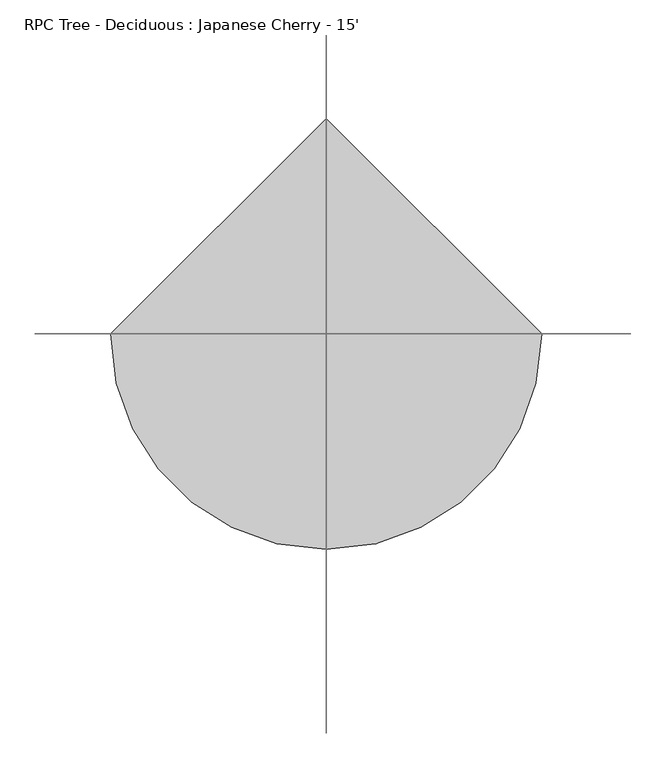
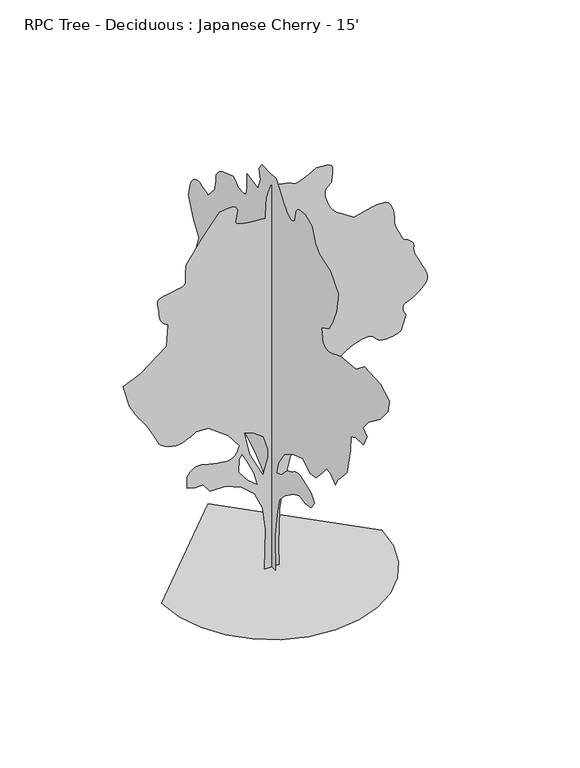
"""IFC4 building model written with IfcOpenShell, lengths in millimetres: geographic element geometry, RPC Tree - Deciduous : Japanese Cherry - 15'."""

from ifc_helpers import new_model, si_unit, origin, place, context, project, spatial, triangles, source, transform, mapped, element, save


def rpc_tree_deciduous_japanese_cherry_15_e499737d(model_context):
    return source(origin(), model_context, "Body", "Tessellation", [
        triangles([(-0.0028028, 75.7657196, 0.0059537), (-0.0028028, -73.2478183, 0.0059537), (-0.0028028, -59.7012251, 399.6312029), (-0.0028028, -100.3410047, 663.7914597), (-0.0028028, -147.7544623, 866.9916292), (-0.0028028, -256.1287339, 982.1375078), (-0.0028028, -418.6863261, 1097.2859299), (-0.0028028, -527.0605977, 1144.6976435), (-0.0028028, -635.434833, 1124.3775902), (-0.0028028, -750.5807842, 1144.6976435), (-0.0028028, -811.5407988, 1232.7519344), (-0.0028028, -750.5807842, 1314.0320023), (-0.0028028, -533.8347845, 1388.5377743), (-0.0028028, -514.9955638, 1387.0189716), (-0.0028028, -496.3341665, 1385.0834793), (-0.0028028, -478.0283798, 1382.3173691), (-0.0028028, -460.2559908, 1378.3091835), (-0.0028028, -443.1947865, 1372.6425236), (-0.0028028, -427.0200471, 1364.9005543), (-0.0028028, -411.9146828, 1354.6719635), (-0.0028028, -396.8067387, 1343.65345), (-0.0028028, -380.6345427, 1333.6991158), (-0.0028028, -363.5733384, 1324.6364422), (-0.0028028, -345.8009494, 1316.2824463), (-0.0028028, -327.4951627, 1308.4643188), (-0.0028028, -308.8337654, 1300.9992222), (-0.0028028, -289.994581, 1293.7118763), (-0.0028028, -188.3942419, 1185.3376774), (-0.0028028, -86.7944115, 1144.6976435), (-0.0028028, -127.4344454, 1286.9377258), (-0.0028028, -242.580869, 1456.2720119), (-0.0028028, -405.140496, 1557.8722057), (-0.0028028, -594.794799, 1618.8321476), (-0.0028028, -730.2607309, 1530.7779293), (-0.0028028, -838.6350025, 1544.3263756), (-0.0028028, -953.7809538, 1666.2439339), (-0.0028028, -1041.8351721, 1774.6181328), (-0.0028028, -1123.1126965, 1767.8439823), (-0.0028028, -1211.1669147, 1686.5663853), (-0.0028028, -1265.3528515, 1781.3922832), (-0.0028028, -1326.3127934, 1849.1240501), (-0.0028028, -1434.6871376, 1964.2723995), (-0.0028028, -1502.4187592, 2269.0726902), (-0.0028028, -1509.193055, 2431.6328259), (-0.0028028, -1604.0214237, 2472.2703163), (-0.0028028, -1753.0332584, 2485.8186172), (-0.0028028, -1813.9932003, 2614.5002975), (-0.0028028, -1739.4874283, 2675.4602394), (-0.0028028, -1841.0874767, 2797.3804138), (-0.0028028, -2071.3792339, 2973.5042564), (-0.0028028, -2220.3935394, 3149.6025192), (-0.0028028, -2247.4851997, 3291.8426743), (-0.0028028, -2078.1535297, 3386.6610146), (-0.0028028, -1766.5790886, 3400.2244308), (-0.0028028, -1610.7931034, 3278.3045471), (-0.0028028, -1312.7669632, 3244.4208595), (-0.0028028, -1272.2845505, 3228.5456657), (-0.0028028, -1232.7519344, 3213.2041603), (-0.0028028, -1195.1115721, 3198.9294502), (-0.0028028, -1160.3186377, 3186.2546425), (-0.0028028, -1129.3153702, 3175.7137161), (-0.0028028, -1103.0517843, 3167.8397781), (-0.0028028, -1082.4726625, 3163.1406464), (-0.0028028, -1064.0500225, 3162.8865921), (-0.0028028, -1044.5580437, 3166.9000099), (-0.0028028, -1025.4242552, 3173.6309944), (-0.0028028, -1008.065867, 3181.5558014), (-0.0028028, -993.907865, 3189.1248161), (-0.0028028, -984.3701477, 3194.789296), (-0.0028028, -980.8726141, 3197.024334), (-0.0028028, -947.0067307, 3359.5844696), (-0.0028028, -1089.2468857, 3434.0828293), (-0.0028028, -1156.9810507, 3542.4645859), (-0.0028028, -1231.4868954, 3718.5628487), (-0.0028028, -1272.127002, 3942.0832169), (-0.0028028, -1116.3410168, 4118.1814796), (-0.0028028, -913.1409199, 4192.7051285), (-0.0028028, -831.8608521, 4267.2034882), (-0.0028028, -770.9007648, 4429.7636238), (-0.0028028, -628.6606825, 4483.9417122), (-0.0028028, -605.4958537, 4483.8402649), (-0.0028028, -582.6891789, 4483.1542603), (-0.0028028, -560.5911455, 4481.2747238), (-0.0028028, -539.5599438, 4477.6426781), (-0.0028028, -519.9511116, 4471.5974075), (-0.0028028, -502.1202959, 4462.6310944), (-0.0028028, -486.4205638, 4450.0836044), (-0.0028028, -473.6824242, 4434.3863068), (-0.0028028, -464.1447433, 4416.5554184), (-0.0028028, -457.2740144, 4396.9467316), (-0.0028028, -452.5343691, 4375.9154572), (-0.0028028, -449.3949532, 4353.8173874), (-0.0028028, -447.3197528, 4331.0083145), (-0.0028028, -445.7805299, 4307.8434494), (-0.0028028, -434.0914178, 4294.9401672), (-0.0028028, -421.9248276, 4283.0531021), (-0.0028028, -408.8133096, 4273.1978897), (-0.0028028, -394.279422, 4266.3398781), (-0.0028028, -377.850701, 4263.5202827), (-0.0028028, -359.0495956, 4265.7303223), (-0.0028028, -337.4062583, 4273.9853416), (-0.0028028, -315.9610193, 4285.9741447), (-0.0028028, -297.7161846, 4298.6995308), (-0.0028028, -282.1358129, 4312.0091835), (-0.0028028, -268.6864885, 4325.8013649), (-0.0028028, -256.8373934, 4339.9237587), (-0.0028028, -246.0563473, 4354.3002068), (-0.0028028, -235.8074452, 4368.8033913), (-0.0028028, -140.9810386, 4497.5054192), (-0.0028028, -80.0209877, 4572.0037788), (-0.0028028, 21.579147, 4565.2219254), (-0.0028028, 184.1389784, 4572.0037788), (-0.0028028, 245.0987749, 4490.7235657), (-0.0028028, 218.0055885, 4375.5852448), (-0.0028028, 265.4200454, 4246.8835075), (-0.0028028, 475.3918765, 4287.5234688), (-0.0028028, 475.3918765, 4138.5014603), (-0.0028028, 476.9514107, 4115.4383331), (-0.0028028, 479.1637756, 4093.1623672), (-0.0028028, 482.6791134, 4072.5630432), (-0.0028028, 488.1502911, 4054.4781006), (-0.0028028, 496.2249435, 4039.6699928), (-0.0028028, 507.5609885, 4029.0273285), (-0.0028028, 522.8060609, 4023.3631393), (-0.0028028, 540.2228757, 4021.2551285), (-0.0028028, 557.6396542, 4020.5691238), (-0.0028028, 575.056469, 4021.0519432), (-0.0028028, 592.4732474, 4022.4995293), (-0.0028028, 609.8900259, 4024.6586998), (-0.0028028, 627.3093842, 4027.2748192), (-0.0028028, 644.726199, 4030.1449928), (-0.0028028, 660.7002239, 4045.9437378), (-0.0028028, 676.7352917, 4060.8791634), (-0.0028028, 692.8896835, 4074.0362091), (-0.0028028, 709.2193554, 4084.5265572), (-0.0028028, 725.7878208, 4091.4607269), (-0.0028028, 742.6534338, 4093.9498192), (-0.0028028, 759.8720776, 4091.1049347), (-0.0028028, 942.7522665, 4030.1449928), (-0.0028028, 968.7009007, 4012.6698967), (-0.0028028, 993.5827394, 3994.8390083), (-0.0028028, 1016.3309875, 3976.2971169), (-0.0028028, 1035.8813931, 3956.6881393), (-0.0028028, 1051.1646172, 3935.6568649), (-0.0028028, 1061.1163353, 3912.8477921), (-0.0028028, 1064.6722956, 3887.9048378), (-0.0028028, 1065.462291, 3862.3526184), (-0.0028028, 1067.6745832, 3837.8921928), (-0.0028028, 1071.0705969, 3814.3209572), (-0.0028028, 1075.4140091, 3791.4610153), (-0.0028028, 1080.4685698, 3769.1088913), (-0.0028028, 1085.9981741, 3747.1381393), (-0.0028028, 1091.7640285, 3725.3447021), (-0.0028028, 1220.4582081, 3583.1045471), (-0.0028028, 1259.5970982, 3600.2497215), (-0.0028028, 1298.4413841, 3615.8705704), (-0.0028028, 1336.691375, 3628.418351), (-0.0028028, 1374.0521759, 3636.343158), (-0.0028028, 1410.2294735, 3638.0956673), (-0.0028028, 1444.9259022, 3632.1521347), (-0.0028028, 1477.8442417, 3616.9629456), (-0.0028028, 1506.4193871, 3593.4931572), (-0.0028028, 1528.9517326, 3564.3086014), (-0.0028028, 1546.4471764, 3530.3996246), (-0.0028028, 1559.9143776, 3492.7059952), (-0.0028028, 1570.361269, 3452.1674812), (-0.0028028, 1578.7941845, 3409.7241417), (-0.0028028, 1586.218586, 3366.3410339), (-0.0028028, 1498.1643677, 3136.0643921), (-0.0028028, 1389.7926395, 2987.0423836), (-0.0028028, 1477.8442417, 2743.2023254), (-0.0028028, 1396.5641739, 2614.5002975), (-0.0028028, 1363.3893093, 2602.8164177), (-0.0028028, 1331.4588455, 2590.6497185), (-0.0028028, 1302.0151485, 2577.543251), (-0.0028028, 1276.3027645, 2563.0144867), (-0.0028028, 1255.5687103, 2546.5806061), (-0.0028028, 1241.0552067, 2527.7820442), (-0.0028028, 1234.0040382, 2506.1385979), (-0.0028028, 1231.6953129, 2483.1135498), (-0.0028028, 1230.4506214, 2460.4416779), (-0.0028028, 1230.0949745, 2438.0692062), (-0.0028028, 1230.4506214, 2415.9330574), (-0.0028028, 1231.339666, 2393.9721886), (-0.0028028, 1232.5842121, 2372.13326), (-0.0028028, 1234.0040382, 2350.3502872), (-0.0028028, 1206.9124506, 2241.9785591), (-0.0028028, 1017.2581112, 2262.2985397), (-0.0028028, 1001.4999161, 2230.5052769), (-0.0028028, 986.9863398, 2199.5401611), (-0.0028028, 974.9594576, 2170.2361359), (-0.0028028, 966.6663591, 2143.4188774), (-0.0028028, 963.3491198, 2119.9211838), (-0.0028028, 966.2523582, 2100.5664059), (-0.0028028, 976.6180773, 2086.1925739), (-0.0028028, 993.4227201, 2074.2646683), (-0.0028028, 1014.0196461, 2062.1005852), (-0.0028028, 1037.2225176, 2050.292149), (-0.0028028, 1061.8478313, 2039.431184), (-0.0028028, 1086.7093952, 2030.1093693), (-0.0028028, 1110.6234879, 2022.9211452), (-0.0028028, 1132.4039898, 2018.4583363), (-0.0028028, 1152.1322187, 2014.567004), (-0.0028028, 1170.7936523, 2008.9003441), (-0.0028028, 1188.5660414, 2001.7526699), (-0.0028028, 1205.6272093, 1993.4190216), (-0.0028028, 1222.157523, 1984.1961834), (-0.0028028, 1238.3297916, 1974.3816662), (-0.0028028, 1254.3241642, 1964.2723995), (-0.0028028, 1410.1126202, 2045.5524673), (-0.0028028, 1454.8979679, 2056.9850544), (-0.0028028, 1498.4412403, 2067.3533169), (-0.0028028, 1539.4952751, 2075.5879887), (-0.0028028, 1576.817997, 2080.6222744), (-0.0028028, 1609.1650051, 2081.3919949), (-0.0028028, 1635.2914627, 2076.8326801), (-0.0028028, 1653.9502075, 2065.8725933), (-0.0028028, 1666.2946575, 2049.9747265), (-0.0028028, 1674.7249569, 2031.5900928), (-0.0028028, 1679.8989143, 2011.1329113), (-0.0028028, 1682.4669262, 1989.0146393), (-0.0028028, 1683.0789528, 1965.6542919), (-0.0028028, 1682.3881519, 1941.4631813), (-0.0028028, 1681.0444839, 1916.8582878), (-0.0028028, 1657.7627655, 1892.3904499), (-0.0028028, 1634.1255455, 1869.1697742), (-0.0028028, 1609.7770317, 1848.4331039), (-0.0028028, 1584.3618679, 1831.4303627), (-0.0028028, 1557.5241165, 1819.4059513), (-0.0028028, 1528.9110374, 1813.5996197), (-0.0028028, 1498.1643677, 1815.2582394), (-0.0028028, 1465.6015297, 1822.4057682), (-0.0028028, 1432.5637207, 1830.9782101), (-0.0028028, 1400.2370602, 1839.0732101), (-0.0028028, 1369.8078129, 1844.8009129), (-0.0028028, 1342.4571568, 1846.2614342), (-0.0028028, 1319.3735367, 1841.5624477), (-0.0028028, 1301.7382759, 1828.8040695), (-0.0028028, 1288.4084209, 1812.3752758), (-0.0028028, 1277.2120113, 1797.7219551), (-0.0028028, 1267.7912201, 1784.5521194), (-0.0028028, 1259.7953419, 1772.5657871), (-0.0028028, 1252.8636429, 1761.4660286), (-0.0028028, 1246.6430923, 1750.9605652), (-0.0028028, 1240.778334, 1740.752322), (-0.0028028, 1263.8618088, 1737.6916077), (-0.0028028, 1286.1172817, 1733.6834221), (-0.0028028, 1306.714135, 1727.7779686), (-0.0028028, 1324.821896, 1719.0302467), (-0.0028028, 1339.6122723, 1706.4901691), (-0.0028028, 1350.2574074, 1689.2105553), (-0.0028028, 1355.9242126, 1666.2439339), (-0.0028028, 1358.2355541, 1639.3300243), (-0.0028028, 1359.4802456, 1610.9912018), (-0.0028028, 1359.8357471, 1581.4687305), (-0.0028028, 1359.4802456, 1550.9989334), (-0.0028028, 1358.591201, 1519.8178425), (-0.0028028, 1357.3466549, 1488.1643967), (-0.0028028, 1355.9242126, 1456.2720119), (-0.0028028, 1321.1312782, 1430.3436527), (-0.0028028, 1286.5720505, 1405.5990875), (-0.0028028, 1252.4876484, 1383.2266159), (-0.0028028, 1219.1146128, 1364.4078518), (-0.0028028, 1186.6915192, 1350.328624), (-0.0028028, 1155.4494581, 1342.1725811), (-0.0028028, 1125.6323828, 1341.1261333), (-0.0028028, 1095.812764, 1344.8167511), (-0.0028028, 1064.5732464, 1349.9322819), (-0.0028028, 1032.1476093, 1356.2316067), (-0.0028028, 998.774501, 1363.478112), (-0.0028028, 964.6902443, 1371.4385273), (-0.0028028, 930.1334873, 1379.8688267), (-0.0028028, 895.3380095, 1388.5377743), (-0.0028028, 692.1378399, 1341.1261333), (-0.0028028, 455.0718596, 1219.2061043), (-0.0028028, 319.6059277, 1144.6976435), (-0.0028028, 163.8189614, 1016.005862), (-0.0028028, 68.9922959, 819.5799156), (-0.0028028, 41.8991095, 541.8713216), (-0.0028028, 68.9922959, 264.1652892), (80.2102203, 0.0002552, 0.0), (-82.349661, 0.0002552, 0.0), (-68.8030678, 0.0002233, 460.5862032), (-102.6694236, 0.000202, 724.7463873), (-190.7229152, 0.0001914, 914.3981833), (-332.9637969, 0.0001914, 1043.0925081), (-509.0697627, 0.0001807, 1117.5983528), (-678.4015417, 0.0001807, 1117.5983528), (-759.684153, 0.0001807, 1219.1984013), (-847.7358278, 0.0001807, 1219.1984013), (-935.7901188, 0.0001807, 1239.5183819), (-935.7901188, 0.0001701, 1368.2127068), (-918.2539072, 0.0001701, 1391.2175526), (-900.0065472, 0.0001701, 1412.9192802), (-880.3392883, 0.0001595, 1432.0150623), (-858.5384388, 0.0001595, 1447.2017807), (-833.8928501, 0.0001595, 1457.1737011), (-805.6936993, 0.0001595, 1460.6307575), (-773.2299831, 0.0001595, 1456.266925), (-734.6829174, 0.0001595, 1446.5108345), (-690.4487715, 0.0001595, 1435.4516258), (-643.1335636, 0.0001701, 1424.2757092), (-595.3460009, 0.0001701, 1414.1639717), (-549.689449, 0.0001701, 1406.3051491), (-508.7725788, 0.0001701, 1401.8804192), (-475.2013721, 0.0001701, 1402.0785175), (-448.544024, 0.0001701, 1408.1415195), (-426.1513865, 0.0001701, 1419.8916744), (-407.3122021, 0.0001595, 1436.3813656), (-391.3152497, 0.0001595, 1456.660651), (-377.4544679, 0.0001595, 1479.7848209), (-365.0135485, 0.0001595, 1504.8039333), (-353.2838139, 0.0001595, 1530.7728424), (-475.2013721, 0.0001488, 1693.3329781), (-698.7215223, 0.0001382, 1855.8931137), (-834.1899977, 0.0001382, 1862.6647934), (-856.0492739, 0.0001382, 1849.6320133), (-878.4419477, 0.0001382, 1836.7771294), (-901.9038877, 0.0001382, 1824.277747), (-926.9610065, 0.0001382, 1812.3092915), (-954.1543322, 0.0001382, 1801.0544552), (-984.01203, 0.0001382, 1790.6861927), (-1017.0701866, 0.0001488, 1781.3847256), (-1055.1015862, 0.0001488, 1778.1664627), (-1097.4002398, 0.0001488, 1784.6638859), (-1140.7656887, 0.0001382, 1798.9792912), (-1182.0000904, 0.0001382, 1819.2206429), (-1217.9005154, 0.0001382, 1843.490237), (-1245.2690483, 0.0001382, 1869.8935673), (-1260.907774, 0.0001382, 1896.5332203), (-1274.5551968, 0.0001382, 1929.7461639), (-1296.2570698, 0.0001276, 1973.9803825), (-1323.2903034, 0.0001276, 2024.4959038), (-1352.9320988, 0.0001276, 2076.5482498), (-1382.45457, 0.0001276, 2125.4025352), (-1409.1321568, 0.0001169, 2166.3195145), (-1430.2420601, 0.0001169, 2194.5592152), (-1448.055217, 0.0001169, 2217.0508656), (-1466.5769062, 0.0001169, 2243.4541958), (-1485.6928905, 0.0001169, 2273.113868), (-1505.2813751, 0.0001169, 2305.3794857), (-1525.2255066, 0.0001063, 2339.6035595), (-1545.4082863, 0.0001063, 2375.12799), (-1565.7080647, 0.0001063, 2411.3051422), (-1640.2164528, 9.57e-05, 2668.7039658), (-1443.7878902, 8.51e-05, 2749.9838882), (-1159.310269, 7.44e-05, 2973.5042564), (-1145.7618954, 5.32e-05, 3217.3190254), (-1165.9447477, 5.32e-05, 3231.9748169), (-1185.2970549, 5.32e-05, 3247.3163223), (-1202.9906696, 5.32e-05, 3264.0804153), (-1218.1951195, 5.32e-05, 3282.9780991), (-1230.0823299, 5.32e-05, 3304.7203766), (-1237.8242992, 5.32e-05, 3330.0188324), (-1240.5902641, 5.32e-05, 3359.5591805), (-1243.0389519, 4.25e-05, 3392.8330215), (-1248.5659401, 4.25e-05, 3427.5294502), (-1254.4511913, 4.25e-05, 3461.7686394), (-1257.9665291, 4.25e-05, 3493.6204742), (-1256.3865383, 4.25e-05, 3521.204837), (-1246.9860947, 4.25e-05, 3542.6169022), (-1227.0419632, 4.25e-05, 3556.002713), (-1192.1092844, 4.25e-05, 3564.4103394), (-1144.1438982, 3.19e-05, 3572.715937), (-1090.0164608, 3.19e-05, 3581.5808029), (-1036.6002445, 3.19e-05, 3591.7915169), (-990.7659056, 3.19e-05, 3603.9835052), (-959.3867163, 3.19e-05, 3618.9186401), (-949.3359489, 3.19e-05, 3637.2829262), (-951.449192, 3.19e-05, 3659.3809959), (-952.1400656, 3.19e-05, 3684.6794518), (-951.644747, 3.19e-05, 3712.6448959), (-950.2045732, 3.19e-05, 3742.718351), (-948.0532511, 2.13e-05, 3774.4175789), (-945.4268852, 2.13e-05, 3807.1836021), (-942.5617258, 2.13e-05, 3840.4830231), (-773.2299831, 1.06e-05, 4084.3233719), (-576.803964, -1.06e-05, 4328.16343), (-534.9980856, -1.06e-05, 4335.1231796), (-494.9117606, -1.06e-05, 4340.3809982), (-458.2595647, -1.06e-05, 4342.2096657), (-426.7635221, -1.06e-05, 4338.8569633), (-402.1382083, -1.06e-05, 4328.6459587), (-386.1031769, -1.06e-05, 4309.850013), (-380.3754742, 0.0, 4280.7416153), (-383.1999384, 0.0, 4247.9503029), (-389.6972889, 0.0, 4219.0450905), (-396.9057878, 0.0, 4193.848082), (-401.8613357, 0.0, 4172.0549355), (-401.6048106, 0.0, 4153.462175), (-393.1720041, 0.0, 4137.8410355), (-373.6038308, 0.0, 4124.9633331), (-343.9238837, 0.0, 4114.5238541), (-307.8431645, 0.0, 4106.2435455), (-266.4335192, 1.06e-05, 4099.7157463), (-220.7586908, 1.06e-05, 4094.6355331), (-171.883967, 1.06e-05, 4090.5971169), (-120.8766607, 1.06e-05, 4087.2697037), (-68.8030678, 1.06e-05, 4084.3233719), (-62.0293897, 0.0, 4267.2034882), (-60.4495079, -1.06e-05, 4293.1367889), (-56.0260951, -1.06e-05, 4318.689299), (-49.2331141, -1.06e-05, 4343.962175), (-40.544273, -1.06e-05, 4369.0065765), (-30.4335416, -1.06e-05, 4393.8733727), (-19.3751868, -1.06e-05, 4418.612851), (-7.8427643, -1.06e-05, 4443.3017509), (38.3857792, -1.06e-05, 4434.5642029), (83.3110485, -1.06e-05, 4425.7249168), (125.6295138, -1.06e-05, 4416.6571564), (164.0381523, -1.06e-05, 4407.2083145), (197.2334371, -1.06e-05, 4397.3022331), (223.9120957, -1.06e-05, 4386.7865959), (242.7705922, -1.06e-05, 4375.5599556), (267.3174405, -1.06e-05, 4372.2834114), (307.2640574, -1.06e-05, 4382.5194145), (355.6256767, -1.06e-05, 4401.5188362), (405.4097383, -1.06e-05, 4424.5566742), (449.6235366, -1.06e-05, 4446.8576385), (481.2770551, -2.13e-05, 4463.7234695), (493.3827115, -2.13e-05, 4470.4035851), (503.1388384, -2.13e-05, 4470.6067703), (528.2975498, -2.13e-05, 4470.3274269), (562.6967946, -2.13e-05, 4468.2699944), (600.177065, -2.13e-05, 4463.1392029), (634.5763098, -1.06e-05, 4453.6142029), (659.7350212, -1.06e-05, 4438.3994339), (669.4911844, -1.06e-05, 4416.1999168), (669.0949877, -1.06e-05, 4390.4698013), (667.9900406, -1.06e-05, 4365.4506889), (666.2907984, -1.06e-05, 4341.0411324), (664.1190559, -1.06e-05, 4317.089106), (661.5918119, -1.06e-05, 4293.4922905), (658.8257017, 0.0, 4270.1245308), (655.9428108, 0.0, 4246.8835075), (638.6835445, 0.0, 4233.6753021), (622.3741476, 0.0, 4219.7308044), (607.9571134, 0.0, 4204.2114029), (596.3848546, 0.0, 4186.4060944), (588.6048426, 0.0, 4165.5271362), (585.5644395, 0.0, 4140.7876579), (588.2111166, 0.0, 4111.3996262), (595.5949319, 1.06e-05, 4078.8367882), (605.8235227, 1.06e-05, 4045.6643944), (618.4244614, 1.06e-05, 4012.9492401), (632.9176901, 1.06e-05, 3981.7834099), (648.8333611, 1.06e-05, 3953.233699), (665.698974, 1.06e-05, 3928.3416138), (683.0370146, 2.13e-05, 3908.1995293), (703.4154945, 2.13e-05, 3889.8099541), (729.1278786, 2.13e-05, 3869.6170006), (759.2802532, 2.13e-05, 3847.9505905), (792.9912043, 2.13e-05, 3825.1159378), (829.3639841, 2.13e-05, 3801.3670967), (867.5148531, 2.13e-05, 3777.0592781), (906.5572374, 2.13e-05, 3752.4212471), (974.48703, 2.13e-05, 3771.0140076), (1040.6997763, 2.13e-05, 3787.8795479), (1103.475959, 2.13e-05, 3801.2909386), (1161.1010027, 2.13e-05, 3809.5712471), (1211.8502306, 2.13e-05, 3810.9682549), (1254.0116833, 2.13e-05, 3803.7800308), (1285.8633728, 2.13e-05, 3786.2793549), (1308.8096466, 2.13e-05, 3757.831382), (1325.9495888, 3.19e-05, 3721.2045479), (1338.1136719, 3.19e-05, 3679.8280037), (1346.1325138, 3.19e-05, 3637.155899), (1350.8315002, 3.19e-05, 3596.6173851), (1353.0438652, 4.25e-05, 3561.641613), (1353.5976105, 4.25e-05, 3535.6827324), (1358.8503422, 4.25e-05, 3507.9969223), (1372.3961723, 4.25e-05, 3469.2870758), (1390.9178616, 4.25e-05, 3425.1418053), (1411.1006413, 5.32e-05, 3381.0982727), (1429.6249466, 5.32e-05, 3342.7442184), (1443.1707767, 5.32e-05, 3315.6423843), (1448.4235085, 5.32e-05, 3305.3808014), (1455.5126106, 5.32e-05, 3302.5614967), (1473.6202263, 5.32e-05, 3294.4079247), (1498.0094353, 5.32e-05, 3281.4031952), (1523.9376492, 5.32e-05, 3264.0042572), (1546.6656223, 5.32e-05, 3242.6936394), (1561.456144, 5.32e-05, 3217.9538704), (1563.5693871, 6.38e-05, 3190.2424805), (1560.9227463, 6.38e-05, 3161.8962456), (1563.9655838, 6.38e-05, 3134.3880409), (1571.7456322, 6.38e-05, 3106.8795456), (1583.3178909, 6.38e-05, 3078.5585999), (1597.7324181, 6.38e-05, 3048.5613029), (1614.0443584, 7.44e-05, 3016.0746231), (1631.3036247, 7.44e-05, 2980.2605301), (1651.0114334, 7.44e-05, 2941.4239471), (1672.8529781, 7.44e-05, 2900.911013), (1693.1526112, 7.44e-05, 2859.5850471), (1708.2377369, 8.51e-05, 2818.2593719), (1714.4404106, 8.51e-05, 2777.7461472), (1708.0801884, 8.51e-05, 2738.9095642), (1685.4894161, 8.51e-05, 2702.5620735), (1655.0603142, 9.57e-05, 2670.8884254), (1626.9983643, 9.57e-05, 2644.9042557), (1600.3587112, 9.57e-05, 2623.6442162), (1574.1941746, 9.57e-05, 2606.1944092), (1547.5546669, 9.57e-05, 2591.5894867), (1519.4951878, 9.57e-05, 2578.8641006), (1489.0634697, 9.57e-05, 2567.103772), (1463.2545799, 9.57e-05, 2553.5147758), (1448.4615875, 9.57e-05, 2536.3646599), (1442.8532089, 9.57e-05, 2516.2632706), (1444.5930737, 0.0001063, 2493.7893517), (1451.8397243, 0.0001063, 2469.5399597), (1462.7592613, 0.0001063, 2444.1069191), (1475.5176395, 0.0001063, 2418.079438), (1421.329232, 0.0001169, 2248.7450066), (1402.2741451, 0.0001169, 2240.1167542), (1382.0913654, 0.0001169, 2231.9607113), (1359.6579964, 0.0001169, 2224.752285), (1333.8491066, 0.0001169, 2218.9661556), (1303.5367126, 0.0001169, 2215.0772942), (1267.5955925, 0.0001169, 2213.5558754), (1224.9032856, 0.0001169, 2214.8791958), (1186.5543182, 0.0001169, 2223.6651421), (1160.2907324, 0.0001169, 2241.2216286), (1139.9504042, 0.0001169, 2263.0426804), (1119.3738258, 0.0001169, 2284.6250839), (1092.3990189, 0.0001169, 2301.470422), (1052.8638594, 0.0001169, 2309.0727196), (994.6089123, 0.0001169, 2302.9309433), (927.2531399, 0.0001169, 2283.7970821), (865.4625074, 0.0001169, 2256.8426228), (810.6645441, 0.0001169, 2224.1985397), (764.2764599, 0.0001169, 2188.0035107), (727.7258566, 0.0001169, 2150.3835686), (702.4274008, 0.0001276, 2113.4772457), (689.8112377, 0.0001276, 2079.4133366), (689.5343651, 0.0001276, 2049.0602474), (699.2092106, 0.0001276, 2021.5520428), (717.179698, 0.0001276, 1996.4136063), (741.7847368, 0.0001276, 1973.172583), (771.3655621, 0.0001382, 1951.3515312), (804.2662428, 0.0001382, 1930.4778053), (838.8229998, 0.0001382, 1910.0790504), (858.9855045, 0.0001382, 1896.9268009), (878.2006107, 0.0001382, 1883.2412991), (895.5183764, 0.0001382, 1868.4914726), (909.9938009, 0.0001382, 1852.1415985), (920.6770878, 0.0001382, 1833.6579884), (926.620693, 0.0001382, 1812.5073898), (926.8772181, 0.0001382, 1788.158876), (924.1721506, 0.0001488, 1758.4790016), (921.8225847, 0.0001488, 1722.4008259), (919.7677683, 0.0001488, 1680.9911442), (917.9516727, 0.0001488, 1635.3142811), (916.3107845, 0.0001595, 1586.4395027), (914.7919092, 0.0001595, 1535.4337498), (913.3288445, 0.0001595, 1483.3585854), (878.4571358, 0.0001595, 1457.529348), (843.3467062, 0.0001595, 1433.4780544), (807.7613056, 0.0001701, 1412.980323), (771.4646839, 0.0001701, 1397.8139523), (734.2231344, 0.0001701, 1389.7570312), (695.792922, 0.0001701, 1390.585033), (655.9428108, 0.0001701, 1402.0785175), (615.8971447, 0.0001701, 1417.3236626), (576.9157305, 0.0001701, 1428.6597439), (538.820781, 0.0001595, 1436.7368671), (501.4395962, 0.0001595, 1442.205574), (464.5917727, 0.0001595, 1445.7209118), (428.0995597, 0.0001595, 1447.9332767), (391.7826267, 0.0001595, 1449.4927746), (276.6366936, 0.0001701, 1374.9868572), (202.1305764, 0.0001807, 1205.6525711), (127.6236689, 0.0001914, 921.1724064), (86.9838894, 0.0002126, 643.4663195), (73.4370464, 0.0002339, 237.0665254), (-95.8962542, 8.51e-05, 1097.2783722), (-41.7096271, 7.44e-05, 1286.9326389), (-41.7096271, 6.38e-05, 1381.7585369), (-89.122576, 5.32e-05, 1544.3186726), (-211.0424234, 5.32e-05, 1632.3728909), (-305.8695931, 5.32e-05, 1666.238847), (-244.9095423, 6.38e-05, 1395.3069832), (-156.8557963, 6.38e-05, 1009.2266247), (-197.4958302, 6.38e-05, 1158.2383867), (-272.003746, 5.32e-05, 1320.7984497), (-326.1896101, 4.25e-05, 1422.3986435), (-360.0554572, 4.25e-05, 1374.9868572), (-366.829644, 5.32e-05, 1225.9725517), (-265.2295592, 6.38e-05, 1097.2783722), (-1212.9170259, 0.0, 0.0045929), (-1180.85205, -277.9194097, 0.0045929), (-1089.5287725, -533.1464181, 0.0045929), (-946.2625174, -758.3633034, 0.0045929), (-758.3633034, -946.2625174, 0.0045929), (-533.1464181, -1089.5287725, 0.0045929), (-277.9194097, -1180.85205, 0.0045929), (5.3e-05, -1212.9170259, 0.0045929), (277.9194097, -1180.85205, 0.0045929), (533.1464181, -1089.5287725, 0.0045929), (758.3633034, -946.2625174, 0.0045929), (946.2625174, -758.3633034, 0.0045929), (1089.5287725, -533.1464181, 0.0045929), (1180.85205, -277.9194097, 0.0045929), (1212.9170259, 0.0001063, 0.0045929), (-0.0001591, 1212.9170259, 0.0045929)], [[38, 39, 40], [115, 116, 117], [1, 2, 3], [280, 1, 3], [279, 280, 3], [279, 3, 4], [278, 279, 4], [278, 4, 5], [186, 187, 188], [277, 278, 5], [46, 47, 48], [45, 46, 48], [277, 5, 6], [185, 186, 188], [10, 11, 12], [9, 10, 12], [9, 12, 13], [8, 9, 13], [8, 13, 14], [8, 14, 15], [8, 15, 16], [8, 16, 17], [8, 17, 18], [8, 18, 19], [8, 19, 20], [8, 20, 21], [7, 8, 21], [7, 21, 22], [7, 22, 23], [7, 23, 24], [7, 24, 25], [7, 25, 26], [6, 7, 26], [6, 26, 27], [6, 27, 28], [277, 6, 28], [277, 28, 29], [51, 52, 53], [50, 51, 53], [50, 53, 54], [50, 54, 55], [49, 50, 55], [49, 55, 56], [48, 49, 56], [48, 56, 57], [45, 48, 57], [44, 45, 57], [44, 57, 58], [44, 58, 59], [44, 59, 60], [44, 60, 61], [44, 61, 62], [44, 62, 63], [276, 277, 29], [276, 29, 30], [184, 185, 188], [183, 184, 188], [44, 63, 64], [115, 117, 118], [111, 112, 113], [111, 113, 114], [182, 183, 188], [109, 110, 111], [109, 111, 114], [108, 109, 114], [108, 114, 115], [107, 108, 115], [106, 107, 115], [105, 106, 115], [104, 105, 115], [115, 118, 119], [170, 171, 172], [170, 172, 173], [170, 173, 174], [170, 174, 175], [74, 75, 76], [74, 76, 77], [73, 74, 77], [72, 73, 77], [71, 72, 77], [258, 259, 260], [181, 182, 188], [78, 79, 80], [170, 175, 176], [103, 104, 115], [78, 80, 81], [44, 64, 65], [275, 276, 30], [275, 30, 31], [274, 275, 31], [78, 81, 82], [78, 82, 83], [78, 83, 84], [78, 84, 85], [78, 85, 86], [78, 86, 87], [78, 87, 88], [78, 88, 89], [78, 89, 90], [78, 90, 91], [78, 91, 92], [78, 92, 93], [78, 93, 94], [78, 94, 95], [78, 95, 96], [71, 77, 78], [71, 78, 96], [71, 96, 97], [71, 97, 98], [71, 98, 99], [71, 99, 100], [115, 119, 120], [180, 181, 188], [38, 40, 41], [223, 224, 225], [33, 34, 35], [33, 35, 36], [33, 36, 37], [102, 103, 115], [179, 180, 188], [44, 65, 66], [170, 176, 177], [71, 100, 101], [43, 44, 66], [42, 43, 66], [41, 42, 66], [38, 41, 66], [37, 38, 66], [33, 37, 66], [33, 66, 67], [33, 67, 68], [33, 68, 69], [33, 69, 70], [32, 33, 70], [31, 32, 70], [274, 31, 70], [273, 274, 70], [273, 70, 71], [273, 71, 101], [273, 101, 102], [273, 102, 115], [273, 115, 120], [273, 120, 121], [273, 121, 122], [273, 122, 123], [273, 123, 124], [273, 124, 125], [273, 125, 126], [273, 126, 127], [273, 127, 128], [273, 128, 129], [273, 129, 130], [273, 130, 131], [272, 273, 131], [271, 272, 131], [270, 271, 131], [269, 270, 131], [268, 269, 131], [268, 131, 132], [268, 132, 133], [268, 133, 134], [167, 168, 169], [257, 258, 260], [257, 260, 261], [256, 257, 261], [256, 261, 262], [255, 256, 262], [255, 262, 263], [254, 255, 263], [254, 263, 264], [254, 264, 265], [254, 265, 266], [254, 266, 267], [254, 267, 268], [253, 254, 268], [252, 253, 268], [251, 252, 268], [250, 251, 268], [249, 250, 268], [248, 249, 268], [247, 248, 268], [246, 247, 268], [245, 246, 268], [166, 167, 169], [165, 166, 169], [164, 165, 169], [163, 164, 169], [162, 163, 169], [161, 162, 169], [160, 161, 169], [159, 160, 169], [158, 159, 169], [157, 158, 169], [156, 157, 169], [155, 156, 169], [154, 155, 169], [154, 169, 170], [154, 170, 177], [153, 154, 177], [153, 177, 178], [153, 178, 179], [153, 179, 188], [222, 223, 225], [222, 225, 226], [221, 222, 226], [220, 221, 226], [219, 220, 226], [218, 219, 226], [217, 218, 226], [216, 217, 226], [215, 216, 226], [214, 215, 226], [213, 214, 226], [212, 213, 226], [212, 226, 227], [212, 227, 228], [212, 228, 229], [212, 229, 230], [212, 230, 231], [211, 212, 231], [211, 231, 232], [211, 232, 233], [210, 211, 233], [209, 210, 233], [209, 233, 234], [209, 234, 235], [209, 235, 236], [209, 236, 237], [209, 237, 238], [209, 238, 239], [209, 239, 240], [208, 209, 240], [208, 240, 241], [207, 208, 241], [206, 207, 241], [206, 241, 242], [205, 206, 242], [204, 205, 242], [204, 242, 243], [203, 204, 243], [202, 203, 243], [202, 243, 244], [201, 202, 244], [201, 244, 245], [201, 245, 268], [200, 201, 268], [199, 200, 268], [198, 199, 268], [197, 198, 268], [196, 197, 268], [195, 196, 268], [194, 195, 268], [153, 188, 189], [153, 189, 190], [152, 153, 190], [152, 190, 191], [151, 152, 191], [136, 137, 138], [135, 136, 138], [135, 138, 139], [134, 135, 139], [134, 139, 140], [134, 140, 141], [134, 141, 142], [134, 142, 143], [134, 143, 144], [134, 144, 145], [134, 145, 146], [134, 146, 147], [134, 147, 148], [134, 148, 149], [134, 149, 150], [134, 150, 151], [134, 151, 191], [134, 191, 192], [134, 192, 193], [268, 134, 193], [194, 268, 193], [583, 580, 581], [574, 281, 575], [580, 583, 584], [573, 574, 575], [583, 581, 575], [580, 584, 585], [572, 573, 575], [582, 583, 575], [582, 575, 281], [571, 572, 575], [571, 575, 576], [281, 282, 283], [570, 571, 576], [570, 576, 577], [344, 345, 346], [290, 291, 292], [406, 407, 408], [570, 577, 578], [290, 292, 293], [289, 290, 293], [289, 293, 294], [289, 294, 295], [289, 295, 296], [289, 296, 297], [289, 297, 298], [289, 298, 299], [289, 299, 300], [289, 300, 301], [289, 301, 302], [289, 302, 303], [288, 289, 303], [287, 288, 303], [287, 303, 304], [287, 304, 305], [287, 305, 306], [286, 287, 306], [286, 306, 307], [286, 307, 308], [286, 308, 309], [569, 570, 578], [554, 555, 556], [405, 406, 408], [343, 344, 346], [512, 513, 514], [511, 512, 514], [511, 514, 515], [511, 515, 516], [511, 516, 517], [510, 511, 517], [510, 517, 518], [510, 518, 519], [510, 519, 520], [510, 520, 521], [510, 521, 522], [510, 522, 523], [510, 523, 524], [509, 510, 524], [509, 524, 525], [508, 509, 525], [434, 435, 436], [342, 343, 346], [507, 508, 525], [507, 525, 526], [405, 408, 409], [404, 405, 409], [403, 404, 409], [403, 409, 410], [402, 403, 410], [401, 402, 410], [400, 401, 410], [400, 410, 411], [399, 400, 411], [399, 411, 412], [399, 412, 413], [399, 413, 414], [399, 414, 415], [377, 378, 379], [341, 342, 346], [341, 346, 347], [340, 341, 347], [339, 340, 347], [338, 339, 347], [337, 338, 347], [336, 337, 347], [335, 336, 347], [334, 335, 347], [333, 334, 347], [377, 379, 380], [377, 380, 381], [377, 381, 382], [377, 382, 383], [377, 383, 384], [377, 384, 385], [377, 385, 386], [377, 386, 387], [377, 387, 388], [377, 388, 389], [377, 389, 390], [377, 390, 391], [376, 377, 391], [376, 391, 392], [375, 376, 392], [374, 375, 392], [373, 374, 392], [372, 373, 392], [372, 392, 393], [371, 372, 393], [370, 371, 393], [369, 370, 393], [369, 393, 394], [369, 394, 395], [369, 395, 396], [332, 333, 347], [369, 396, 397], [426, 427, 428], [426, 428, 429], [425, 426, 429], [425, 429, 430], [424, 425, 430], [424, 430, 431], [423, 424, 431], [423, 431, 432], [422, 423, 432], [422, 432, 433], [421, 422, 433], [420, 421, 433], [419, 420, 433], [418, 419, 433], [418, 433, 434], [418, 434, 436], [418, 436, 437], [418, 437, 438], [418, 438, 439], [417, 418, 439], [417, 439, 440], [416, 417, 440], [416, 440, 441], [415, 416, 441], [399, 415, 441], [399, 441, 442], [399, 442, 443], [399, 443, 444], [399, 444, 445], [399, 445, 446], [399, 446, 447], [399, 447, 448], [399, 448, 449], [369, 397, 398], [331, 332, 347], [368, 369, 398], [360, 361, 362], [359, 360, 362], [359, 362, 363], [358, 359, 363], [358, 363, 364], [357, 358, 364], [357, 364, 365], [356, 357, 365], [355, 356, 365], [355, 365, 366], [354, 355, 366], [353, 354, 366], [352, 353, 366], [351, 352, 366], [350, 351, 366], [349, 350, 366], [348, 349, 366], [348, 366, 367], [348, 367, 368], [348, 368, 398], [347, 348, 398], [347, 398, 399], [347, 399, 449], [347, 449, 450], [347, 450, 451], [347, 451, 452], [331, 347, 452], [331, 452, 453], [331, 453, 454], [331, 454, 455], [331, 455, 456], [330, 331, 456], [329, 330, 456], [328, 329, 456], [327, 328, 456], [326, 327, 456], [325, 326, 456], [324, 325, 456], [323, 324, 456], [322, 323, 456], [321, 322, 456], [320, 321, 456], [319, 320, 456], [318, 319, 456], [317, 318, 456], [316, 317, 456], [315, 316, 456], [314, 315, 456], [314, 456, 457], [314, 457, 458], [314, 458, 459], [314, 459, 460], [314, 460, 461], [314, 461, 462], [314, 462, 463], [314, 463, 464], [314, 464, 465], [314, 465, 466], [314, 466, 467], [314, 467, 468], [314, 468, 469], [314, 469, 470], [314, 470, 471], [314, 471, 472], [314, 472, 473], [314, 473, 474], [314, 474, 475], [314, 475, 476], [314, 476, 477], [314, 477, 478], [314, 478, 479], [314, 479, 480], [314, 480, 481], [314, 481, 482], [314, 482, 483], [314, 483, 484], [314, 484, 485], [314, 485, 486], [314, 486, 487], [314, 487, 488], [314, 488, 489], [314, 489, 490], [314, 490, 491], [314, 491, 492], [314, 492, 493], [314, 493, 494], [314, 494, 495], [314, 495, 496], [314, 496, 497], [314, 497, 498], [314, 498, 499], [314, 499, 500], [314, 500, 501], [314, 501, 502], [580, 585, 586], [554, 556, 557], [553, 554, 557], [553, 557, 558], [553, 558, 559], [553, 559, 560], [553, 560, 561], [553, 561, 562], [553, 562, 563], [552, 553, 563], [552, 563, 564], [551, 552, 564], [550, 551, 564], [550, 564, 565], [549, 550, 565], [549, 565, 566], [548, 549, 566], [547, 548, 566], [546, 547, 566], [545, 546, 566], [544, 545, 566], [543, 544, 566], [542, 543, 566], [541, 542, 566], [540, 541, 566], [539, 540, 566], [538, 539, 566], [538, 566, 567], [537, 538, 567], [537, 567, 568], [537, 568, 569], [537, 569, 578], [536, 537, 578], [535, 536, 578], [535, 578, 579], [534, 535, 579], [534, 579, 580], [533, 534, 580], [532, 533, 580], [507, 526, 527], [506, 507, 527], [531, 532, 580], [506, 527, 528], [530, 531, 580], [281, 283, 284], [582, 281, 284], [582, 284, 285], [582, 285, 286], [588, 582, 286], [587, 588, 286], [587, 286, 309], [586, 587, 309], [586, 309, 310], [586, 310, 311], [586, 311, 312], [586, 312, 313], [580, 586, 313], [580, 313, 314], [530, 580, 314], [529, 530, 314], [502, 503, 504], [502, 504, 505], [314, 502, 505], [529, 314, 505], [529, 505, 506], [529, 506, 528], [603, 604, 589], [602, 603, 589], [602, 589, 590], [601, 602, 590], [601, 590, 591], [601, 591, 592], [600, 601, 592], [599, 600, 592], [599, 592, 593], [599, 593, 594], [599, 594, 595], [599, 595, 596], [599, 596, 597], [599, 597, 598]], closed=False),
    ])


if __name__ == "__main__":
    model = new_model("IFC4")
    model_context = context("Model", 3, world=origin())
    ifc_project = project(units=[si_unit("LENGTHUNIT", "METRE", prefix="MILLI")], contexts=[model_context])
    site = spatial("IfcSite", under=ifc_project)
    building = spatial("IfcBuilding", under=site)
    placement = place(None, origin())
    rpc_tree_deciduous_japanese_cherry_15_shape = rpc_tree_deciduous_japanese_cherry_15_e499737d(model_context)
    element("IfcGeographicElement", 1, ObjectType="RPC Tree - Deciduous : Japanese Cherry - 15'", at=placement, inside=building, context=model_context, shape_type="MappedRepresentation", body=[
        mapped(rpc_tree_deciduous_japanese_cherry_15_shape, transform((0.0, 0.0, 0.0), x_axis=(1.0, 0.0, 0.0), y_axis=(0.0, 1.0, 0.0), z_axis=(0.0, 0.0, 1.0))),
    ])
    save(model, "model.ifc")

# Revit data of these elements
# Type "RPC Tree - Deciduous : Japanese Cherry - 15'"
#   built-in parameter 1005198 = "{2, 15},{39, RPC-16-FXGW-2MQ0-PN7K-A000-ST1L-LVER-AU},{1, 0},{1, 0},{2, 13},{1, 8},{5, Color},{1, 0},{1, 0},{3, 0.8},{3, 0.8},{3, 0.8},{1, 8},{7, BBoxMin},{1, 0},{1, 0},{1, 0},{1, 0},{1, 0},{1, 8},{7, BBoxMax},{1, 0},{1, 0},{1, 0},{1, 0},{1, 0},{2, 11},{9, RPCTypeId},{1, 0},{1, 0},{39, RPC-16-FXGW-2MQ0-PN7K-A000-ST1L-LVER-AU},{1, 6},{14, RPCPlantHeight},{1, 0},{1, 0},{2, 15},{2, 11},{7, keyword},{1, 0},{1, 0},{34, :RPCs:Trees [General]:Geometry:RPC},{2, 11},{8, category},{1, 0},{1, 0},{15, Trees [General]},{2, 11},{12, LocalizedUID},{1, 0},{1, 0},{25, Japanese Flowering Cherry},{2, 14},{6, Height},{1, 0},{1, 0},{2, 15},{1, 2},{16, Cast Reflections},{1, 0},{1, 0},{1, 0},{1, 2},{12, Cast Shadows},{1, 0},{1, 0},{1, 1},{1, 2},{9, Lock View},{1, 0},{1, 0},{1, 0},{1, 4},{5, ViewC},{1, 0},{1, 0},{1, 0},{21, assetlibrary_base.fbx},{1, 5},"
#   built-in parameter 1005195 = "RPC-16-FXGW-2MQ0-PN7K-A000-ST1L-LVER-AU"
#   Type Comments = "Japanese Cherry"
#   Assembly Code = "G2050500"
#   Height = 15' - 0"
#   Default Elevation = 0
